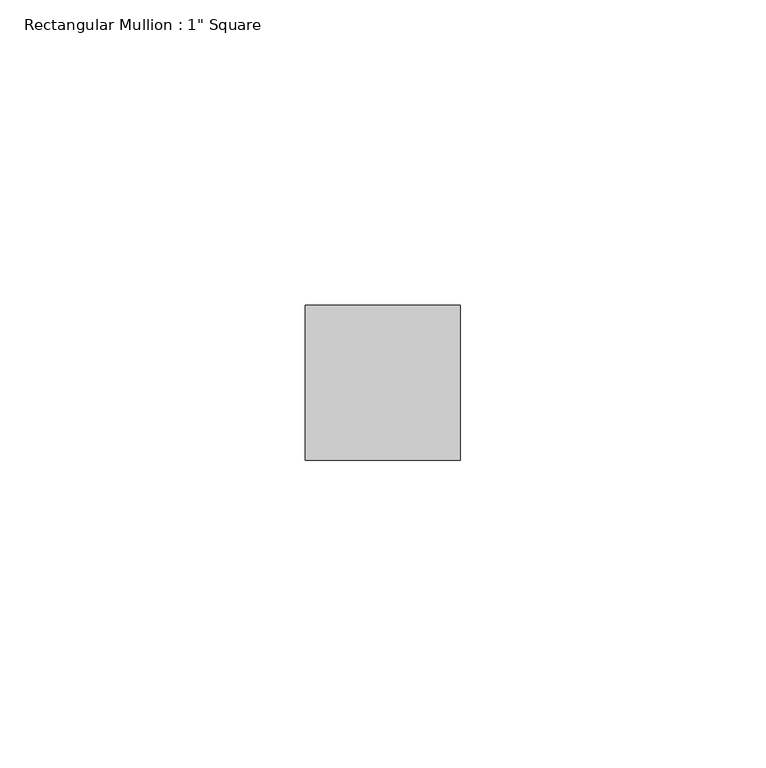
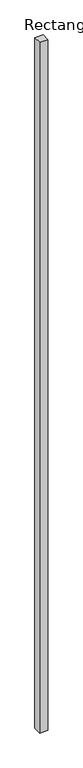
"""IFC4 building model written with IfcOpenShell, lengths in millimetres: member geometry."""

from ifc_helpers import new_model, si_unit, frame, origin, place, context, project, spatial, polyline, outline, extrude, source, transform, mapped, element, save


def member_f9b59f6e(model_context):
    return source(origin(), model_context, "Body", "SweptSolid", [
        extrude(outline(polyline([(12.7, 12.7), (12.7, -12.7), (-12.7, -12.7), (-12.7, 12.7), (12.7, 12.7)])), frame((0.0, 0.0, -2287.5875), z_axis=(0.0, 0.0, 1.0), x_axis=(1.0, 0.0, 0.0)), (0.0, 0.0, 1.0), 2287.5875),
    ])


if __name__ == "__main__":
    model = new_model("IFC4")
    model_context = context("Model", 3, world=origin())
    ifc_project = project(units=[si_unit("LENGTHUNIT", "METRE", prefix="MILLI")], contexts=[model_context])
    site = spatial("IfcSite", under=ifc_project)
    building = spatial("IfcBuilding", under=site)
    placement = place(None, origin())
    member_shape = member_f9b59f6e(model_context)
    element("IfcMember", 1, ObjectType="Rectangular Mullion : 1\" Square", at=placement, inside=building, context=model_context, shape_type="MappedRepresentation", body=[
        mapped(member_shape, transform((0.0, 0.0, 0.0), x_axis=(1.0, 0.0, 0.0), y_axis=(0.0, 1.0, 0.0), z_axis=(0.0, 0.0, 1.0))),
    ])
    save(model, "model.ifc")

# Revit data of these elements
# Type "Rectangular Mullion : 1\" Square"
#   built-in parameter 1007304 = 0.0833333 (stored number, unit not read)
#   built-in parameter 1007301 = 0.0416667 (stored number, unit not read)
#   built-in parameter 1007300 = 0.0416667 (stored number, unit not read)
# Element 1 (IfcMember, "Rectangular Mullion : 1\" Square")
#   Materials on its faces: "black"
# Materials
#   "black": class "Generic", colour RGB 120 120 120, transparency 0, Cost = 0
